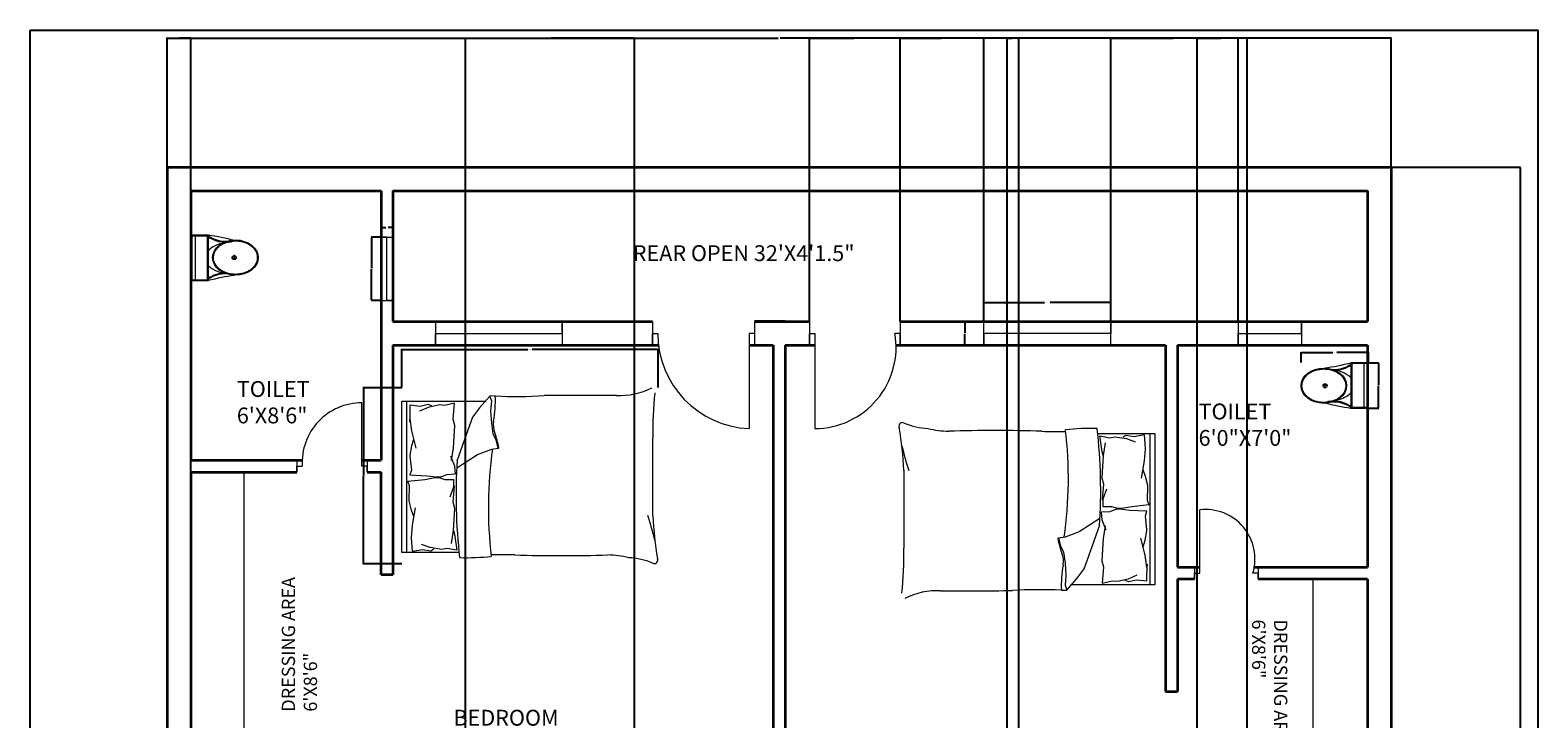
# Model space of a CAD drawing. Units: inches. Extents: x 2460 to 3031, y 933 to 2010.
# Tile 7 of 7: x 2460 to 3031, y 1749 to 2010. Entities that reach past the tile are written whole.
import ezdxf

# ---------------------------------------------------------------- set-up
doc = ezdxf.new("R2010")
doc.units = ezdxf.units.IN
for name, color, linetype, lineweight in [('A-ANNO-DIMS', 2, 'Continuous', 18), ('A-ANNO-TTLB', 7, 'Continuous', 25), ('A-AREA-IDEN', 7, 'Continuous', 18), ('A-DOOR', 4, 'Continuous', 18), ('A-FLOR-CASE', 9, 'Continuous', 18), ('A-FLOR-FIXT', 8, 'Continuous', 18), ('A-FURN', 8, 'Continuous', 18), ('A-GLAZ', 4, 'Continuous', 18), ('A-WALL', 7, 'Continuous', 35), ('C-PROP', 7, 'Continuous', 35)]:
    doc.layers.add(name, color=color, linetype=linetype, lineweight=lineweight)
doc.styles.get("Standard").update_dxf_attribs({"font": 'arial.ttf'})
doc.dimstyles.get("Standard").update_dxf_attribs({"dimtxt": 0.18, "dimasz": 0.18, "dimexe": 0.18, "dimexo": 0.0625, "dimgap": 0.09, "dimtad": 0, "dimtih": 1, "dimtoh": 1, "dimdec": 4, "dimzin": 0, "dimdsep": 46, "dimtxsty": 'Standard', "dimcen": 0.09, "dimadec": 0, "dimazin": 0, "dimtfac": 1, "dimtdec": 4, "dimtofl": 0, "dimtmove": 0, "dimatfit": 3, "dimfxl": 1, "dimtolj": 1, "dimtzin": 0, "dimarcsym": 0})

# ---------------------------------------------------------------- blocks, each defined once
blk = doc.blocks.new('A$C31115884')
for p, q in [((258, 466), (258, 523)), ((283, 498), (223, 498)), ((0, 200), (0, 0)), ((520, 200), (0, 200)), ((10, 190), (10, 10)), ((510, 190), (10, 190)), ((510, 10), (510, 190)), ((520, 0), (520, 200)), ((510, 54), (0, 54)), ((10, 10), (510, 10)), ((0, 0), (520, 0))]:
    blk.add_line(p, q)
blk.add_circle((256, 496), 23.6)
for centre, radius, start, end in [((2778, -205), 2807, 165.4549, 171.7133), ((-295, 403), 365, 324.2091, 9.3499), ((-295, 403), 375, 324.2091, 9.3499), ((384, 406), 293, 190.2774, 224.1564), ((139, 406), 293, 315.8436, 2.6563), ((806, 403), 375, 179.2036, 215.7909), ((806, 403), 365, 170.6501, 215.7909), ((3237, 905), 2807, 188.2867, 194.5451)]:
    blk.add_arc(centre, radius, start, end)
blk.add_ellipse((256, 510), major_axis=(0, -261), ratio=0.772727)
blk.add_open_spline([(256, 259), (263, 259), (270, 260), (288, 262), (299, 265), (320, 273), (330, 278), (350, 291), (360, 299), (378, 316), (386, 326), (402, 347), (409, 358), (421, 383), (427, 395), (436, 422), (440, 436), (445, 465), (447, 480), (448, 509), (448, 524), (445, 553), (443, 568), (436, 596), (432, 610), (422, 636), (416, 649), (402, 672), (395, 683), (379, 703), (370, 712), (351, 728), (341, 735), (321, 746), (310, 751), (289, 757), (278, 759), (256, 761), (245, 761), (223, 757), (212, 754), (191, 746), (181, 741), (161, 728), (151, 720), (133, 703), (125, 693), (110, 672), (103, 660), (90, 636), (85, 623), (76, 596), (72, 582), (67, 553), (66, 538), (64, 509), (65, 494), (68, 465), (70, 450), (77, 422), (81, 408), (91, 382), (97, 370), (111, 346), (118, 335), (135, 316), (144, 307), (162, 291), (172, 284), (193, 273), (203, 269), (225, 262), (236, 260), (250, 259), (253, 259), (256, 259)], degree=3, knots=[0, 0, 0, 0, 0.110105, 0.110105, 0.285049, 0.285049, 0.459994, 0.459994, 0.634938, 0.634938, 0.809882, 0.809882, 0.984827, 0.984827, 1.159771, 1.159771, 1.334715, 1.334715, 1.50966, 1.50966, 1.684604, 1.684604, 1.859549, 1.859549, 2.034493, 2.034493, 2.209437, 2.209437, 2.384382, 2.384382, 2.559326, 2.559326, 2.73427, 2.73427, 2.909215, 2.909215, 3.084159, 3.084159, 3.259103, 3.259103, 3.434048, 3.434048, 3.608992, 3.608992, 3.783936, 3.783936, 3.958881, 3.958881, 4.133825, 4.133825, 4.30877, 4.30877, 4.483714, 4.483714, 4.658658, 4.658658, 4.833603, 4.833603, 5.008547, 5.008547, 5.183491, 5.183491, 5.358436, 5.358436, 5.53338, 5.53338, 5.708324, 5.708324, 5.883269, 5.883269, 6.058213, 6.058213, 6.233158, 6.233158, 6.283185, 6.283185, 6.283185, 6.283185])
blk = doc.blocks.new('BED-DOUBLE')
for p, q in [((75.16, 62.38), (96.87, 62.38)), ((76.95, 55.42), (76.08, 61.53)), ((76.08, 61.53), (79.9, 60.84)), ((78.14, 58.9), (77.34, 54.06)), ((79.9, 60.84), (81.8, 61.19)), ((81.8, 61.19), (86.14, 60.49)), ((85.96, 61.71), (84.75, 61.01)), ((89.08, 61.19), (85.96, 61.71)), ((86.14, 60.49), (89.43, 59.28)), ((92.9, 61.88), (89.08, 61.19)), ((92.87, 61.87), (93.27, 56.74)), ((95.03, 62.38), (95.03, 5.09)), ((96.87, 62.38), (96.87, 5.09)), ((77.34, 54.06), (76.82, 45.66)), ((77.34, 54.06), (76.95, 55.42)), ((92.9, 52.03), (91.68, 45.45)), ((93.24, 56.62), (92.9, 52.03)), ((93.27, 56.74), (93.24, 56.62)), ((1.87, 48.49), (1.87, 18.98)), ((92.38, 48.74), (93.24, 46.31)), ((93.24, 46.31), (94.11, 42.85)), ((76.82, 45.66), (77.49, 43.31)), ((77.49, 43.31), (77, 37.16)), ((77.37, 37.65), (78.68, 41.42)), ((94.11, 42.46), (93.94, 37.13)), ((94.11, 42.85), (94.11, 42.46)), ((77.37, 34.71), (77.37, 37.65)), ((80.59, 34.71), (77.37, 34.71)), ((82.84, 34.01), (80.59, 34.71)), ((88.22, 34.71), (84.4, 34.01)), ((94.63, 35.4), (88.22, 34.71)), ((93.94, 37.13), (94.63, 35.4)), ((76.03, 30.27), (68.25, 25.25)), ((79.83, 32.82), (76.62, 32.62)), ((76.62, 32.62), (76.8, 29.68)), ((76.8, 29.68), (78.34, 26)), ((82.03, 33.66), (79.83, 32.82)), ((83.59, 33.75), (82.03, 33.66)), ((84.4, 34.01), (82.84, 34.01)), ((87.44, 33.3), (83.59, 33.75)), ((93.88, 33.01), (87.44, 33.3)), ((93.3, 31.24), (93.88, 33.01)), ((93.81, 25.93), (93.3, 31.24)), ((62.87, 23.21), (60.45, 22.84)), ((60.45, 22.84), (61.2, 19.86)), ((68.25, 25.25), (62.87, 23.21)), ((72.52, 17.82), (76.03, 27.82)), ((78.14, 27.51), (77.34, 22.68)), ((93.18, 22.03), (93.83, 25.54)), ((93.83, 25.54), (93.81, 25.93)), ((61.2, 19.86), (62.31, 17.45)), ((62.31, 17.45), (62.87, 13.37)), ((70.1, 11.14), (72.52, 17.82)), ((77.34, 22.68), (76.82, 14.27)), ((93.19, 16.3), (91.57, 22.8)), ((92.47, 19.55), (93.18, 22.03)), ((62.87, 13.37), (63.24, 8.72)), ((76.82, 14.27), (77.49, 11.92)), ((77.49, 11.92), (77, 5.77)), ((93.82, 11.75), (93.19, 16.3)), ((93.81, 6.47), (93.92, 12.95)), ((93.92, 12.95), (93.82, 11.75)), ((63.24, 8.72), (62.87, 5.01)), ((63.61, 3.17), (67.51, 7.61)), ((67.51, 7.61), (70.1, 11.14)), ((77, 5.77), (80.77, 6.7)), ((80.77, 6.7), (82.69, 6.47)), ((82.69, 6.47), (86.97, 7.43)), ((86.88, 6.21), (85.62, 6.83)), ((89.96, 6.93), (86.88, 6.21)), ((86.97, 7.43), (90.18, 8.85)), ((93.81, 6.47), (89.96, 6.93)), ((61.52, 3.07), (63.61, 3.17, 4.64)), ((62.87, 5.01), (63.61, 3.17)), ((96.87, 5.09), (64.97, 5.09))]:
    blk.add_line(p, q)
for centre, radius, start, end in [((1.3, 65.24), 1.31, 56.1736, 203.4781), ((-143.9, 40.86), 145.97, 2.9958, 9.4091), ((12.62, 92.52), 28.25, 247.9751, 266.652), ((19.53, 98.8), 35.53, 256.0648, 268.9113), ((36.19, -514.68), 578.22, 88.22771, 91.71854), ((59.5, 267.13), 203.94, 268.4762, 271.0082), ((-90.53, 45.26), 154.68, 351.7845, 6.9006), ((72.78, -35.55), 99.87, 88.7218, 95.604), ((-121.38, 40.94), 197.77, 356.0865, 6.7821), ((125.3, 87.2), 127.63, 193.3832, 197.7053), ((60.38, 22.63), 0.221, 70.2464, 181.1377), ((-157.62, 17.21), 159.5, 354.4998, 0.6351), ((95.1, 29.2), 35.55, 190.6617, 199.8806), ((104.85, 5.01), 43.38, 169.8763, 182.5657), ((54.83, 14.11), 7.46, 348.6608, 23.7384), ((14.55, -24.75), 27.65, 87.4714, 116.4681), ((15.56, 5471.89), 5469.02, 270.00217, 270.28689), ((53.34, -151.96), 155.25, 86.9791, 93.8365)]:
    blk.add_arc(centre, radius, start, end)
blk = doc.blocks.new('WIN-24-PARTITION')
for p, q in [((2.25, 24), (0, 24)), ((0, 24), (4.5, 24)), ((2.25, 0), (2.25, 24)), ((0, 0), (4.5, 0)), ((4.5, 0), (2.25, 0))]:
    blk.add_line(p, q)
blk = doc.blocks.new('WIN-48')
for p, q in [((0, 9), (0, 0)), ((48, 4.5), (48, 9)), ((48, 9), (48, 0)), ((0, 0), (0, 4.5)), ((0, 4.5), (48, 4.5))]:
    blk.add_line(p, q)
blk = doc.blocks.new('*D12')
at = {"layer": 'A-ANNO-DIMS', "color": 0, "lineweight": -2, "transparency": 16777216}
for p, q in [((2600.56, 1874.46), (2600.56, 1889.13)), ((2600.74, 1888.95), (2648.25, 1888.95)), ((2697.38, 1888.95), (2649.88, 1888.95)), ((2697.56, 1874.46), (2697.56, 1889.13))]:
    blk.add_line(p, q, dxfattribs=at)
at = {"layer": 'A-ANNO-DIMS', "color": 0, "transparency": 16777216}
for points in [[(2600.74, 1888.98), (2600.74, 1888.92), (2600.56, 1888.95)], [(2697.38, 1888.98), (2697.38, 1888.92), (2697.56, 1888.95)]]:
    blk.add_solid(points, dxfattribs=at)
at = {"layer": 'Defpoints', "color": 0, "transparency": 16777216}
for p in [(2600.56, 1888.95), (2600.56, 1874.4), (2697.56, 1874.4)]:
    blk.add_point(p, dxfattribs=at)
at = {"layer": 'A-ANNO-DIMS', "color": 0, "transparency": 16777216, "insert": (2649.06, 1888.95), "char_height": 0.18, "attachment_point": 5}
blk.add_mtext('\\A1;BED 97 TYP.', dxfattribs=at)
blk = doc.blocks.new('*D13')
at = {"layer": 'A-ANNO-DIMS', "color": 0, "lineweight": -2, "transparency": 16777216}
for p, q in [((2600.5, 1874.4), (2585.83, 1874.4)), ((2586.01, 1874.22), (2586.01, 1841.26)), ((2586.01, 1807.93), (2586.01, 1840.89)), ((2600.5, 1807.75), (2585.83, 1807.75))]:
    blk.add_line(p, q, dxfattribs=at)
at = {"layer": 'A-ANNO-DIMS', "color": 0, "transparency": 16777216}
for points in [[(2585.98, 1874.22), (2586.04, 1874.22), (2586.01, 1874.4)], [(2585.98, 1807.93), (2586.04, 1807.93), (2586.01, 1807.75)]]:
    blk.add_solid(points, dxfattribs=at)
at = {"layer": 'Defpoints', "color": 0, "transparency": 16777216}
for p in [(2600.56, 1874.4), (2586.01, 1807.75), (2600.56, 1807.75)]:
    blk.add_point(p, dxfattribs=at)
at = {"layer": 'A-ANNO-DIMS', "color": 0, "transparency": 16777216, "insert": (2586.01, 1841.08), "char_height": 0.18, "attachment_point": 5}
blk.add_mtext('\\A1;67 TYP.', dxfattribs=at)
blk = doc.blocks.new('*D14')
at = {"layer": 'A-ANNO-DIMS', "color": 0, "lineweight": -2, "transparency": 16777216}
for p, q in [((2941.02, 1883.97), (2941.02, 1887.91)), ((2941.2, 1887.73), (2952.98, 1887.73)), ((2966.32, 1887.73), (2954.54, 1887.73)), ((2966.5, 1883.97), (2966.5, 1887.91))]:
    blk.add_line(p, q, dxfattribs=at)
at = {"layer": 'A-ANNO-DIMS', "color": 0, "transparency": 16777216}
for points in [[(2941.2, 1887.76), (2941.2, 1887.7), (2941.02, 1887.73)], [(2966.32, 1887.76), (2966.32, 1887.7), (2966.5, 1887.73)]]:
    blk.add_solid(points, dxfattribs=at)
at = {"layer": 'Defpoints', "color": 0, "transparency": 16777216}
for p in [(2941.02, 1887.73), (2941.02, 1883.91), (2966.5, 1883.91)]:
    blk.add_point(p, dxfattribs=at)
at = {"layer": 'A-ANNO-DIMS', "color": 0, "transparency": 16777216, "insert": (2953.76, 1887.73), "char_height": 0.18, "attachment_point": 5}
blk.add_mtext('\\A1;WC 25 TYP.', dxfattribs=at)
blk = doc.blocks.new('*D15')
at = {"layer": 'A-ANNO-DIMS', "color": 0, "lineweight": -2, "transparency": 16777216}
for p, q in [((2966.56, 1883.91), (2970.5, 1883.91)), ((2970.32, 1883.73), (2970.32, 1875.49)), ((2970.32, 1866.9), (2970.32, 1875.13)), ((2966.56, 1866.72), (2970.5, 1866.72))]:
    blk.add_line(p, q, dxfattribs=at)
at = {"layer": 'A-ANNO-DIMS', "color": 0, "transparency": 16777216}
for points in [[(2970.29, 1883.73), (2970.35, 1883.73), (2970.32, 1883.91)], [(2970.29, 1866.9), (2970.35, 1866.9), (2970.32, 1866.72)]]:
    blk.add_solid(points, dxfattribs=at)
at = {"layer": 'Defpoints', "color": 0, "transparency": 16777216}
for p in [(2966.5, 1883.91), (2970.32, 1883.91), (2966.5, 1866.72)]:
    blk.add_point(p, dxfattribs=at)
at = {"layer": 'A-ANNO-DIMS', "color": 0, "transparency": 16777216, "insert": (2970.32, 1875.31), "char_height": 0.18, "attachment_point": 5}
blk.add_mtext('\\A1;17 TYP.', dxfattribs=at)
blk = doc.blocks.new('*D26')
at = {"layer": 'A-ANNO-DIMS', "color": 0, "lineweight": -2, "transparency": 16777216}
for p, q in [((2592.61, 1931.46), (2588.89, 1931.46)), ((2589.07, 1931.28), (2589.07, 1919.64)), ((2589.07, 1907.64), (2589.07, 1919.27)), ((2592.61, 1907.46), (2588.89, 1907.46))]:
    blk.add_line(p, q, dxfattribs=at)
at = {"layer": 'A-ANNO-DIMS', "color": 0, "transparency": 16777216}
for points in [[(2589.04, 1931.28), (2589.1, 1931.28), (2589.07, 1931.46)], [(2589.04, 1907.64), (2589.1, 1907.64), (2589.07, 1907.46)]]:
    blk.add_solid(points, dxfattribs=at)
at = {"layer": 'Defpoints', "color": 0, "transparency": 16777216}
for p in [(2589.07, 1931.46), (2592.67, 1931.46), (2592.67, 1907.46)]:
    blk.add_point(p, dxfattribs=at)
at = {"layer": 'A-ANNO-DIMS', "color": 0, "transparency": 16777216, "insert": (2589.07, 1919.46), "char_height": 0.18, "attachment_point": 5}
blk.add_mtext('\\A1;WINDOW 24 TYP.', dxfattribs=at)
blk = doc.blocks.new('*D27')
at = {"layer": 'A-ANNO-DIMS', "color": 0, "lineweight": -2, "transparency": 16777216}
for p, q in [((2592.67, 1931.52), (2592.67, 1935.24)), ((2597.17, 1931.52), (2597.17, 1935.24)), ((2592.85, 1935.06), (2594.46, 1935.06)), ((2596.99, 1935.06), (2595.38, 1935.06))]:
    blk.add_line(p, q, dxfattribs=at)
at = {"layer": 'A-ANNO-DIMS', "color": 0, "transparency": 16777216}
for points in [[(2592.85, 1935.09), (2592.85, 1935.03), (2592.67, 1935.06)], [(2596.99, 1935.09), (2596.99, 1935.03), (2597.17, 1935.06)]]:
    blk.add_solid(points, dxfattribs=at)
at = {"layer": 'Defpoints', "color": 0, "transparency": 16777216}
for p in [(2592.67, 1931.46), (2597.17, 1935.06), (2597.17, 1931.46)]:
    blk.add_point(p, dxfattribs=at)
at = {"layer": 'A-ANNO-DIMS', "color": 0, "transparency": 16777216, "insert": (2594.92, 1935.06), "char_height": 0.18, "attachment_point": 5}
blk.add_mtext('\\A1;5 TYP.', dxfattribs=at)
blk = doc.blocks.new('*D28')
at = {"layer": 'A-ANNO-DIMS', "color": 0, "lineweight": -2, "transparency": 16777216}
for p, q in [((2820.93, 1899.55), (2820.93, 1906.86)), ((2821.11, 1906.68), (2843.81, 1906.68)), ((2868.75, 1906.68), (2846.05, 1906.68)), ((2868.93, 1899.55), (2868.93, 1906.86))]:
    blk.add_line(p, q, dxfattribs=at)
at = {"layer": 'A-ANNO-DIMS', "color": 0, "transparency": 16777216}
for points in [[(2821.11, 1906.71), (2821.11, 1906.65), (2820.93, 1906.68)], [(2868.75, 1906.71), (2868.75, 1906.65), (2868.93, 1906.68)]]:
    blk.add_solid(points, dxfattribs=at)
at = {"layer": 'Defpoints', "color": 0, "transparency": 16777216}
for p in [(2820.93, 1906.68), (2820.93, 1899.48), (2868.93, 1899.48)]:
    blk.add_point(p, dxfattribs=at)
at = {"layer": 'A-ANNO-DIMS', "color": 0, "transparency": 16777216, "insert": (2844.93, 1906.68), "char_height": 0.18, "attachment_point": 5}
blk.add_mtext('\\A1;WINDOW 48 TYP.', dxfattribs=at)
blk = doc.blocks.new('*D29')
at = {"layer": 'A-ANNO-DIMS', "color": 0, "lineweight": -2, "transparency": 16777216}
for p, q in [((2820.86, 1899.48), (2813.55, 1899.48)), ((2813.73, 1899.3), (2813.73, 1895.16)), ((2820.86, 1890.48), (2813.55, 1890.48)), ((2813.73, 1890.66), (2813.73, 1894.8))]:
    blk.add_line(p, q, dxfattribs=at)
at = {"layer": 'A-ANNO-DIMS', "color": 0, "transparency": 16777216}
for points in [[(2813.7, 1899.3), (2813.76, 1899.3), (2813.73, 1899.48)], [(2813.7, 1890.66), (2813.76, 1890.66), (2813.73, 1890.48)]]:
    blk.add_solid(points, dxfattribs=at)
at = {"layer": 'Defpoints', "color": 0, "transparency": 16777216}
for p in [(2820.93, 1899.48), (2813.73, 1890.48), (2820.93, 1890.48)]:
    blk.add_point(p, dxfattribs=at)
at = {"layer": 'A-ANNO-DIMS', "color": 0, "transparency": 16777216, "insert": (2813.73, 1894.98), "char_height": 0.18, "attachment_point": 5}
blk.add_mtext('\\A1;9 TYP.', dxfattribs=at)
blk = doc.blocks.new('*D32')
at = {"layer": 'A-ANNO-DIMS', "color": 0, "lineweight": -2, "transparency": 16777216}
for p, q in [((2511.67, 1958.05), (2511.67, 2006.96)), ((2511.85, 2006.78), (2743.02, 2006.78)), ((2974.99, 2006.78), (2743.82, 2006.78)), ((2975.17, 1958.05), (2975.17, 2006.96))]:
    blk.add_line(p, q, dxfattribs=at)
at = {"layer": 'A-ANNO-DIMS', "color": 0, "transparency": 16777216}
for points in [[(2511.85, 2006.81), (2511.85, 2006.75), (2511.67, 2006.78)], [(2974.99, 2006.81), (2974.99, 2006.75), (2975.17, 2006.78)]]:
    blk.add_solid(points, dxfattribs=at)
at = {"layer": 'Defpoints', "color": 0, "transparency": 16777216}
for p in [(2975.17, 2006.78), (2511.67, 1957.98), (2975.17, 1957.98)]:
    blk.add_point(p, dxfattribs=at)
at = {"layer": 'A-ANNO-DIMS', "color": 0, "transparency": 16777216, "insert": (2743.42, 2006.78), "char_height": 0.18, "attachment_point": 5}
blk.add_mtext('\\A1;463.5', dxfattribs=at)
blk = doc.blocks.new('*D33')
at = {"layer": 'A-ANNO-DIMS', "color": 0, "lineweight": -2, "transparency": 16777216}
for p, q in [((2975.23, 1957.98), (3024.15, 1957.98)), ((3023.97, 1957.8), (3023.97, 1507.16)), ((3023.97, 1056.16), (3023.97, 1506.8)), ((2975.23, 1055.98), (3024.15, 1055.98))]:
    blk.add_line(p, q, dxfattribs=at)
at = {"layer": 'A-ANNO-DIMS', "color": 0, "transparency": 16777216}
for points in [[(3023.94, 1957.8), (3024, 1957.8), (3023.97, 1957.98)], [(3023.94, 1056.16), (3024, 1056.16), (3023.97, 1055.98)]]:
    blk.add_solid(points, dxfattribs=at)
at = {"layer": 'Defpoints', "color": 0, "transparency": 16777216}
for p in [(2975.17, 1957.98), (3023.97, 1957.98), (2975.17, 1055.98)]:
    blk.add_point(p, dxfattribs=at)
at = {"layer": 'A-ANNO-DIMS', "color": 0, "transparency": 16777216, "insert": (3023.97, 1506.98), "char_height": 0.18, "attachment_point": 5}
blk.add_mtext('\\A1;902', dxfattribs=at)
blk = doc.blocks.new('*D40')
at = {"layer": 'A-ANNO-DIMS', "color": 0, "lineweight": -2, "transparency": 16777216}
for p, q in [((2511.67, 1056.05), (2511.67, 2006.96)), ((2511.85, 2006.78), (2516.02, 2006.78)), ((2520.49, 2006.78), (2516.32, 2006.78)), ((2520.67, 1056.05), (2520.67, 2006.96))]:
    blk.add_line(p, q, dxfattribs=at)
at = {"layer": 'A-ANNO-DIMS', "color": 0, "transparency": 16777216}
for points in [[(2511.85, 2006.81), (2511.85, 2006.75), (2511.67, 2006.78)], [(2520.49, 2006.81), (2520.49, 2006.75), (2520.67, 2006.78)]]:
    blk.add_solid(points, dxfattribs=at)
at = {"layer": 'Defpoints', "color": 0, "transparency": 16777216}
for p in [(2520.67, 2006.78), (2511.67, 1055.98), (2520.67, 1055.98)]:
    blk.add_point(p, dxfattribs=at)
at = {"layer": 'A-ANNO-DIMS', "color": 0, "transparency": 16777216, "insert": (2516.17, 2006.78), "char_height": 0.18, "attachment_point": 5}
blk.add_mtext('\\A1;9', dxfattribs=at)
blk = doc.blocks.new('*D41')
at = {"layer": 'A-ANNO-DIMS', "color": 0, "lineweight": -2, "transparency": 16777216}
for p, q in [((2829.67, 1599.92), (2829.67, 2006.96)), ((2829.85, 2006.78), (2831.66, 2006.78)), ((2833.99, 2006.78), (2832.18, 2006.78)), ((2834.17, 1599.92), (2834.17, 2006.96))]:
    blk.add_line(p, q, dxfattribs=at)
at = {"layer": 'A-ANNO-DIMS', "color": 0, "transparency": 16777216}
for points in [[(2829.85, 2006.81), (2829.85, 2006.75), (2829.67, 2006.78)], [(2833.99, 2006.81), (2833.99, 2006.75), (2834.17, 2006.78)]]:
    blk.add_solid(points, dxfattribs=at)
at = {"layer": 'Defpoints', "color": 0, "transparency": 16777216}
for p in [(2834.17, 2006.78), (2829.67, 1599.86), (2834.17, 1599.86)]:
    blk.add_point(p, dxfattribs=at)
at = {"layer": 'A-ANNO-DIMS', "color": 0, "transparency": 16777216, "insert": (2831.92, 2006.78), "char_height": 0.18, "attachment_point": 5}
blk.add_mtext('\\A1;4.5', dxfattribs=at)
blk = doc.blocks.new('*D44')
at = {"layer": 'A-ANNO-DIMS', "color": 0, "lineweight": -2, "transparency": 16777216}
for p, q in [((2624.64, 1348.55), (2624.64, 2006.96)), ((2624.82, 2006.78), (2656.26, 2006.78)), ((2688.49, 2006.78), (2657.05, 2006.78)), ((2688.67, 1348.55), (2688.67, 2006.96))]:
    blk.add_line(p, q, dxfattribs=at)
at = {"layer": 'A-ANNO-DIMS', "color": 0, "transparency": 16777216}
for points in [[(2624.82, 2006.81), (2624.82, 2006.75), (2624.64, 2006.78)], [(2688.49, 2006.81), (2688.49, 2006.75), (2688.67, 2006.78)]]:
    blk.add_solid(points, dxfattribs=at)
at = {"layer": 'Defpoints', "color": 0, "transparency": 16777216}
for p in [(2688.67, 2006.78), (2624.64, 1348.48), (2688.67, 1348.48)]:
    blk.add_point(p, dxfattribs=at)
at = {"layer": 'A-ANNO-DIMS', "color": 0, "transparency": 16777216, "insert": (2656.65, 2006.78), "char_height": 0.18, "attachment_point": 5}
blk.add_mtext('\\A1;64.03', dxfattribs=at)
blk = doc.blocks.new('*D46')
at = {"layer": 'A-ANNO-DIMS', "color": 0, "lineweight": -2, "transparency": 16777216}
for p, q in [((2868.93, 1899.55), (2868.93, 2006.96)), ((2869.11, 2006.78), (2892.64, 2006.78)), ((2916.97, 2006.78), (2893.44, 2006.78)), ((2917.15, 1899.55), (2917.15, 2006.96))]:
    blk.add_line(p, q, dxfattribs=at)
at = {"layer": 'A-ANNO-DIMS', "color": 0, "transparency": 16777216}
for points in [[(2869.11, 2006.81), (2869.11, 2006.75), (2868.93, 2006.78)], [(2916.97, 2006.81), (2916.97, 2006.75), (2917.15, 2006.78)]]:
    blk.add_solid(points, dxfattribs=at)
at = {"layer": 'Defpoints', "color": 0, "transparency": 16777216}
for p in [(2917.15, 2006.78), (2868.93, 1899.48), (2917.15, 1899.48)]:
    blk.add_point(p, dxfattribs=at)
at = {"layer": 'A-ANNO-DIMS', "color": 0, "transparency": 16777216, "insert": (2893.04, 2006.78), "char_height": 0.18, "attachment_point": 5}
blk.add_mtext('\\A1;48.22', dxfattribs=at)
blk = doc.blocks.new('*D47')
at = {"layer": 'A-ANNO-DIMS', "color": 0, "lineweight": -2, "transparency": 16777216}
for p, q in [((2754.88, 1899.55), (2754.88, 2006.96)), ((2755.06, 2006.78), (2771.66, 2006.78)), ((2789.06, 2006.78), (2772.45, 2006.78)), ((2789.24, 1899.55), (2789.24, 2006.96))]:
    blk.add_line(p, q, dxfattribs=at)
at = {"layer": 'A-ANNO-DIMS', "color": 0, "transparency": 16777216}
for points in [[(2755.06, 2006.81), (2755.06, 2006.75), (2754.88, 2006.78)], [(2789.06, 2006.81), (2789.06, 2006.75), (2789.24, 2006.78)]]:
    blk.add_solid(points, dxfattribs=at)
at = {"layer": 'Defpoints', "color": 0, "transparency": 16777216}
for p in [(2789.24, 2006.78), (2754.88, 1899.48), (2789.24, 1899.48)]:
    blk.add_point(p, dxfattribs=at)
at = {"layer": 'A-ANNO-DIMS', "color": 0, "transparency": 16777216, "insert": (2772.06, 2006.78), "char_height": 0.18, "attachment_point": 5}
blk.add_mtext('\\A1;34.36', dxfattribs=at)
blk = doc.blocks.new('*D48')
at = {"layer": 'A-ANNO-DIMS', "color": 0, "lineweight": -2, "transparency": 16777216}
for p, q in [((2789.24, 1899.55), (2789.24, 2006.96)), ((2789.42, 2006.78), (2804.69, 2006.78)), ((2820.75, 2006.78), (2805.48, 2006.78)), ((2820.93, 1899.55), (2820.93, 2006.96))]:
    blk.add_line(p, q, dxfattribs=at)
at = {"layer": 'A-ANNO-DIMS', "color": 0, "transparency": 16777216}
for points in [[(2789.42, 2006.81), (2789.42, 2006.75), (2789.24, 2006.78)], [(2820.75, 2006.81), (2820.75, 2006.75), (2820.93, 2006.78)]]:
    blk.add_solid(points, dxfattribs=at)
at = {"layer": 'Defpoints', "color": 0, "transparency": 16777216}
for p in [(2820.93, 2006.78), (2789.24, 1899.48), (2820.93, 1899.48)]:
    blk.add_point(p, dxfattribs=at)
at = {"layer": 'A-ANNO-DIMS', "color": 0, "transparency": 16777216, "insert": (2805.08, 2006.78), "char_height": 0.18, "attachment_point": 5}
blk.add_mtext('\\A1;31.69', dxfattribs=at)
blk = doc.blocks.new('*D49')
at = {"layer": 'A-ANNO-DIMS', "color": 0, "lineweight": -2, "transparency": 16777216}
for p, q in [((2901.62, 1437.52), (2901.62, 2006.96)), ((2901.8, 2006.78), (2910.66, 2006.78)), ((2920.43, 2006.78), (2911.57, 2006.78)), ((2920.61, 1437.52), (2920.61, 2006.96))]:
    blk.add_line(p, q, dxfattribs=at)
at = {"layer": 'A-ANNO-DIMS', "color": 0, "transparency": 16777216}
for points in [[(2901.8, 2006.81), (2901.8, 2006.75), (2901.62, 2006.78)], [(2920.43, 2006.81), (2920.43, 2006.75), (2920.61, 2006.78)]]:
    blk.add_solid(points, dxfattribs=at)
at = {"layer": 'Defpoints', "color": 0, "transparency": 16777216}
for p in [(2920.61, 2006.78), (2901.62, 1437.46), (2920.61, 1437.46)]:
    blk.add_point(p, dxfattribs=at)
at = {"layer": 'A-ANNO-DIMS', "color": 0, "transparency": 16777216, "insert": (2911.11, 2006.78), "char_height": 0.18, "attachment_point": 5}
blk.add_mtext('\\A1;18.996', dxfattribs=at)

msp = doc.modelspace()

# ---------------------------------------------------------------- linework, layer by layer
at = {"layer": 'A-ANNO-TTLB'}
msp.add_lwpolyline([(2459.8083, 2009.7942), (3030.6598, 2009.7942), (3030.6598, 936.3732), (2459.8083, 936.3732)], close=True, dxfattribs=at)
at = {"layer": 'A-DOOR'}
for p, q in [((2695.4544, 1899.4828), (2695.4544, 1890.4828)), ((2734.0149, 1899.4828), (2734.0149, 1890.4828)), ((2754.8751, 1899.4828), (2754.8751, 1890.4828)), ((2789.2373, 1899.4828), (2789.2373, 1890.4828)), ((2695.4544, 1890.4828), (2695.4544, 1894.9828)), ((2695.4544, 1894.9828), (2697.4544, 1894.9828)), ((2734.0149, 1894.9828), (2732.0149, 1894.9828)), ((2732.0149, 1894.9828), (2732.0149, 1858.9828)), ((2754.8751, 1890.4828), (2754.8751, 1894.9828)), ((2754.8751, 1894.9828), (2756.8751, 1894.9828)), ((2756.8751, 1894.9828), (2756.8751, 1858.9828)), ((2789.2373, 1894.9828), (2787.2373, 1894.9828)), ((2789.2373, 1890.4828), (2789.2373, 1894.9828)), ((2585.4123, 1844.7328), (2585.4123, 1868.7328)), ((2560.8286, 1846.9828), (2560.8286, 1842.4828)), ((2560.8286, 1842.4828), (2560.8286, 1844.7328)), ((2560.8286, 1844.7328), (2562.8286, 1844.7328)), ((2587.4123, 1844.7328), (2585.4123, 1844.7328)), ((2587.4123, 1846.9828), (2587.4123, 1842.4828)), ((2587.4123, 1842.4828), (2587.4123, 1844.7328)), ((2902.6174, 1804.2328), (2902.6174, 1828.2328)), ((2900.6174, 1806.4828), (2900.6174, 1801.9828)), ((2900.6174, 1801.9828), (2900.6174, 1804.2328)), ((2900.6174, 1804.2328), (2902.6174, 1804.2328)), ((2924.7836, 1804.2328), (2922.7836, 1804.2328)), ((2924.7836, 1806.4828), (2924.7836, 1801.9828)), ((2924.7836, 1801.9828), (2924.7836, 1804.2328))]:
    msp.add_line(p, q, dxfattribs=at)
for centre, radius, start, end in [((2733.4844, 1894.9828), 36.03, 180, 267.662476), ((2756.8751, 1889.7864), 30.8036, 270, 9.711885), ((2585.4123, 1846.1073), 22.6255, 90, 183.482826), ((2904.8082, 1809.6012), 18.76, 343.371657, 96.706243)]:
    msp.add_arc(centre, radius, start, end, dxfattribs=at)
at = {"layer": 'A-FLOR-CASE'}
for p, q in [((2540.7485, 1842.4828), (2540.7485, 1740.4828)), ((2945.476, 1801.9828), (2945.476, 1714.4828))]:
    msp.add_line(p, q, dxfattribs=at)
at = {"layer": 'A-GLAZ'}
for p, q in [((2917.1507, 1899.4828), (2917.1507, 1890.4828)), ((2941.1507, 1894.9828), (2941.1507, 1899.4828)), ((2941.1507, 1899.4828), (2941.1507, 1890.4828)), ((2917.1507, 1890.4828), (2917.1507, 1894.9828)), ((2917.1507, 1894.9828), (2941.1507, 1894.9828))]:
    msp.add_line(p, q, dxfattribs=at)
at = {"layer": 'A-WALL'}
for p, q in [((2520.6684, 1948.9828), (2592.6684, 1948.9828)), ((2520.6684, 1948.9828), (2520.6684, 1846.9828)), ((2592.6684, 1948.9828), (2592.6684, 1846.9828)), ((2597.1684, 1948.9828), (2597.1684, 1899.4828)), ((2597.1684, 1899.4828), (2695.4544, 1899.4828)), ((2745.6684, 1899.4828), (2734.0149, 1899.4828)), ((2734.0149, 1899.4828), (2754.8751, 1899.4828)), ((2789.2373, 1899.4828), (2966.1684, 1899.4828)), ((2597.1684, 1890.4828), (2697.7365, 1890.4828)), ((2597.1684, 1890.4828), (2597.1684, 1842.4828)), ((2732.0149, 1890.4828), (2741.1684, 1890.4828)), ((2734.0149, 1890.4828), (2741.1684, 1890.4828)), ((2741.1684, 1890.4828), (2741.1684, 1714.4828)), ((2745.6684, 1890.4828), (2745.6684, 1714.4828)), ((2745.6684, 1890.4828), (2756.8751, 1890.4828)), ((2787.6709, 1890.4828), (2889.6684, 1890.4828)), ((2889.6684, 1890.4828), (2889.6684, 1759.3898)), ((2894.1684, 1890.4828), (2894.1684, 1806.4828)), ((2894.1684, 1890.4828), (2966.1684, 1890.4828)), ((2894.1684, 1890.4828), (2894.1684, 1806.4828)), ((2966.1684, 1890.4828), (2966.1684, 1806.4828)), ((2520.6684, 1846.9828), (2562.8037, 1846.9828)), ((2585.4123, 1846.9828), (2592.6684, 1846.9828)), ((2520.6684, 1842.4828), (2560.8286, 1842.4828)), ((2520.6684, 1842.4828), (2520.6684, 1635.4828)), ((2587.4123, 1842.4828), (2592.6684, 1842.4828)), ((2592.6684, 1803.5384), (2592.6684, 1842.4828)), ((2597.1684, 1842.4828), (2597.1684, 1803.5384)), ((2894.1684, 1806.4828), (2902.6174, 1806.4828)), ((2923.3072, 1806.4828), (2966.1684, 1806.4828)), ((2597.1684, 1803.5384), (2592.6684, 1803.5384)), ((2894.1684, 1801.9828), (2894.1684, 1759.3898)), ((2900.6174, 1801.9828), (2894.1684, 1801.9828)), ((2966.1684, 1801.9828), (2924.7836, 1801.9828)), ((2966.1684, 1801.9828), (2966.1684, 1504.4828)), ((2889.6684, 1759.3898), (2894.1684, 1759.3898))]:
    msp.add_line(p, q, dxfattribs=at)
at = {"layer": 'C-PROP'}
for p, q in [((2511.6684, 1957.9828), (2511.6684, 1055.9828)), ((2511.6684, 1957.9828), (2511.6684, 1055.9828)), ((2511.6684, 1957.9828), (2975.1684, 1957.9828)), ((2975.1684, 1957.9828), (2975.1684, 1055.9828)), ((2597.1684, 1948.9828), (2966.1684, 1948.9828)), ((2966.1684, 1948.9828), (2966.1684, 1899.4828))]:
    msp.add_line(p, q, dxfattribs=at)

# ---------------------------------------------------------------- block references
at = {"layer": 'A-FLOR-FIXT', "xscale": 0.0330640103915726, "yscale": 0.0330640103915726, "zscale": 0.0330640103915726}
for p, rotation in [((2520.6684, 1932.1604), 269.9999999999999), ((2966.4991, 1866.7158), 89.99999999999991)]:
    msp.add_blockref('A$C31115884', p, dxfattribs=dict(at, rotation=rotation))
at = {"layer": 'A-FURN', "rotation": 180}
msp.add_blockref('BED-DOUBLE', (2697.4361, 1874.402), dxfattribs=at)
at = {"layer": 'A-FURN'}
msp.add_blockref('BED-DOUBLE', (2788.758, 1794.683), dxfattribs=at)
at = {"layer": 'A-GLAZ'}
for name, p in [('WIN-24-PARTITION', (2592.668, 1907.458)), ('WIN-48', (2613.226, 1890.483))]:
    msp.add_blockref(name, p, dxfattribs=at)
at = {"layer": 'A-GLAZ', "rotation": 180}
msp.add_blockref('WIN-48', (2868.9273, 1899.4826), dxfattribs=at)

# ---------------------------------------------------------------- texts
at = {"layer": 'A-AREA-IDEN', "char_height": 6, "attachment_point": 1}
for s, width, insert in [('REAR OPEN 32\'X4\'1.5"', 218.671944, (2687.9655, 1928.3614)), ('TOILET\\P6\'X8\'6"', 128.563737, (2538.0618, 1876.9434)), ('TOILET\\P6\'0"X7\'0"', 57.978148, (2902.1985, 1868.4334)), ('BEDROOM\\P12\'8"X14\'0"', 68.258258, (2620.0635, 1752.504))]:
    msp.add_mtext_dynamic_manual_height_columns(s, width=width, gutter_width=12.5, heights=[0], dxfattribs=dict(at, insert=insert))
at = {"layer": 'A-AREA-IDEN', "char_height": 5, "attachment_point": 1}
for width, insert, rotation in [(104.31142, (2555.0911, 1751.7922), 90), (124.82599, (2935.8013, 1786.6763), 270)]:
    msp.add_mtext_dynamic_manual_height_columns('DRESSING AREA\\P6\'X8\'6"', width=width, gutter_width=12.5, heights=[0], dxfattribs=dict(at, insert=insert, rotation=rotation))

# ---------------------------------------------------------------- dimensions: what is measured, and where the dimension line sits
at = {"layer": 'A-ANNO-DIMS'}
for base, p1, p2, override, picture, middle in [((2975.1684, 2006.7823), (2511.6684, 1957.9828), (2975.1684, 1957.9828), {"dimdec": 1, "dimlfac": 1, "dimrnd": 0, "dimzin": 0, "dimdsep": 46, "dimlunit": 2}, '*D32', (2743.4184, 2006.7823)), ((2520.6684, 2006.7823), (2511.6684, 1055.9828), (2520.6684, 1055.9828), {"dimdec": 0, "dimlfac": 1, "dimrnd": 0, "dimzin": 0, "dimdsep": 46, "dimlunit": 2}, '*D40', (2516.1684, 2006.7823)), ((2688.6684, 2006.7823), (2624.6394, 1348.4828), (2688.6684, 1348.4828), {"dimdec": 2, "dimlfac": 1, "dimrnd": 0, "dimzin": 0, "dimdsep": 46, "dimlunit": 2}, '*D44', (2656.6539, 2006.7823)), ((2789.2373, 2006.7823), (2754.8751, 1899.4828), (2789.2373, 1899.4828), {"dimdec": 2, "dimlfac": 1, "dimrnd": 0, "dimzin": 0, "dimdsep": 46, "dimlunit": 2}, '*D47', (2772.0562, 2006.7823)), ((2820.9268, 2006.7823), (2789.2373, 1899.4828), (2820.9268, 1899.4828), {"dimdec": 2, "dimlfac": 1, "dimrnd": 0, "dimzin": 0, "dimdsep": 46, "dimlunit": 2}, '*D48', (2805.082, 2006.7823)), ((2834.1684, 2006.7823), (2829.6684, 1599.86), (2834.1684, 1599.86), {"dimdec": 1, "dimlfac": 1, "dimrnd": 0, "dimzin": 0, "dimdsep": 46, "dimlunit": 2}, '*D41', (2831.9184, 2006.7823)), ((2917.1507, 2006.7823), (2868.9268, 1899.4828), (2917.1507, 1899.4828), {"dimdec": 2, "dimlfac": 1, "dimrnd": 0, "dimzin": 0, "dimdsep": 46, "dimlunit": 2}, '*D46', (2893.0388, 2006.7823)), ((2920.6119, 2006.7823), (2901.6162, 1437.4597), (2920.6119, 1437.4597), {"dimdec": 3, "dimlfac": 1, "dimrnd": 0, "dimzin": 0, "dimdsep": 46, "dimlunit": 2}, '*D49', (2911.1141, 2006.7823))]:
    dim = msp.add_linear_dim(base=base, p1=p1, p2=p2, dimstyle='Standard', override=override, dxfattribs=at)
    dim.commit()
    dim.dimension.update_dxf_attribs({"geometry": picture, "text_midpoint": middle})
dim = msp.add_linear_dim(base=(3023.9679, 1957.9828), p1=(2975.1684, 1055.9828), p2=(2975.1684, 1957.9828), angle=90, dimstyle='Standard', override={"dimdec": 0, "dimlfac": 1, "dimrnd": 0, "dimzin": 0, "dimdsep": 46, "dimlunit": 2}, dxfattribs=at)
dim.commit()
dim.dimension.update_dxf_attribs({"geometry": '*D33', "text_midpoint": (3023.9679, 1506.9828)})
dim = msp.add_linear_dim(base=(2597.1684287001, 1935.0579536479), p1=(2592.6684287001, 1931.4579536479), p2=(2597.1684287001, 1931.4579536479), text='<> TYP.', dimstyle='Standard', override={"dimdec": 0, "dimlfac": 1, "dimrnd": 0, "dimzin": 0, "dimdsep": 46, "dimlunit": 2}, dxfattribs=at)
dim.commit()
dim.dimension.update_dxf_attribs({"geometry": '*D27', "text_midpoint": (2594.9184287001, 1935.0579536479)})
for base, p1, p2, angle, text, picture, middle in [((2589.0684, 1931.458), (2592.6684, 1907.458), (2592.6684, 1931.458), 90, 'WINDOW <> TYP.', '*D26', (2589.0684, 1919.458)), ((2820.9268, 1906.6828), (2868.9268, 1899.4828), (2820.9268, 1899.4828), 180, 'WINDOW <> TYP.', '*D28', (2844.9268, 1906.6828)), ((2813.7268, 1890.4828), (2820.9268, 1899.4828), (2820.9268, 1890.4828), 270, '<> TYP.', '*D29', (2813.7268, 1894.9828)), ((2600.5638, 1888.9513), (2697.5626, 1874.4015), (2600.5638, 1874.4015), 180, 'BED <> TYP.', '*D12', (2649.0632, 1888.9513)), ((2941.0209, 1887.7308), (2966.4991, 1883.9091), (2941.0209, 1883.9091), 180, 'WC <> TYP.', '*D14', (2953.76, 1887.7308)), ((2970.3208, 1883.9091), (2966.4991, 1866.7158), (2966.4991, 1883.9091), 90, '<> TYP.', '*D15', (2970.3208, 1875.3125)), ((2586.014, 1807.75), (2600.5638, 1874.4015), (2600.5638, 1807.75), 270, '<> TYP.', '*D13', (2586.014, 1841.0757))]:
    dim = msp.add_linear_dim(base=base, p1=p1, p2=p2, angle=angle, text=text, dimstyle='Standard', override={"dimdec": 0, "dimlfac": 1, "dimrnd": 0, "dimzin": 0, "dimdsep": 46, "dimlunit": 2}, dxfattribs=at)
    dim.commit()
    dim.dimension.update_dxf_attribs({"geometry": picture, "text_midpoint": middle})

doc.saveas('drawing.dxf')
